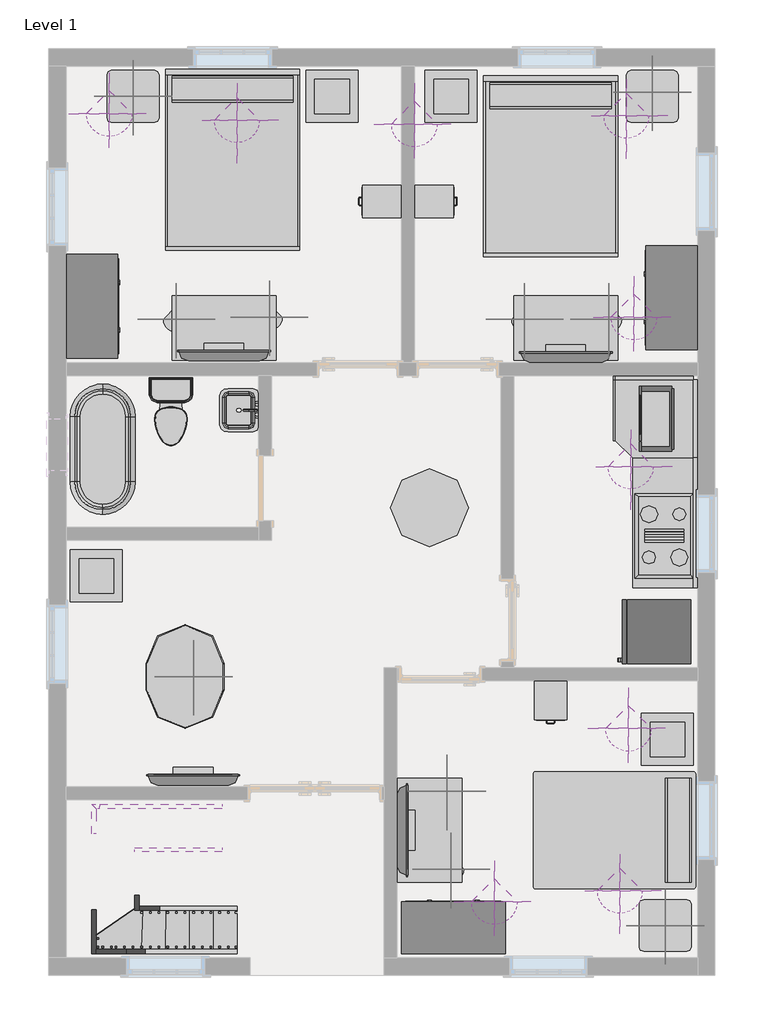
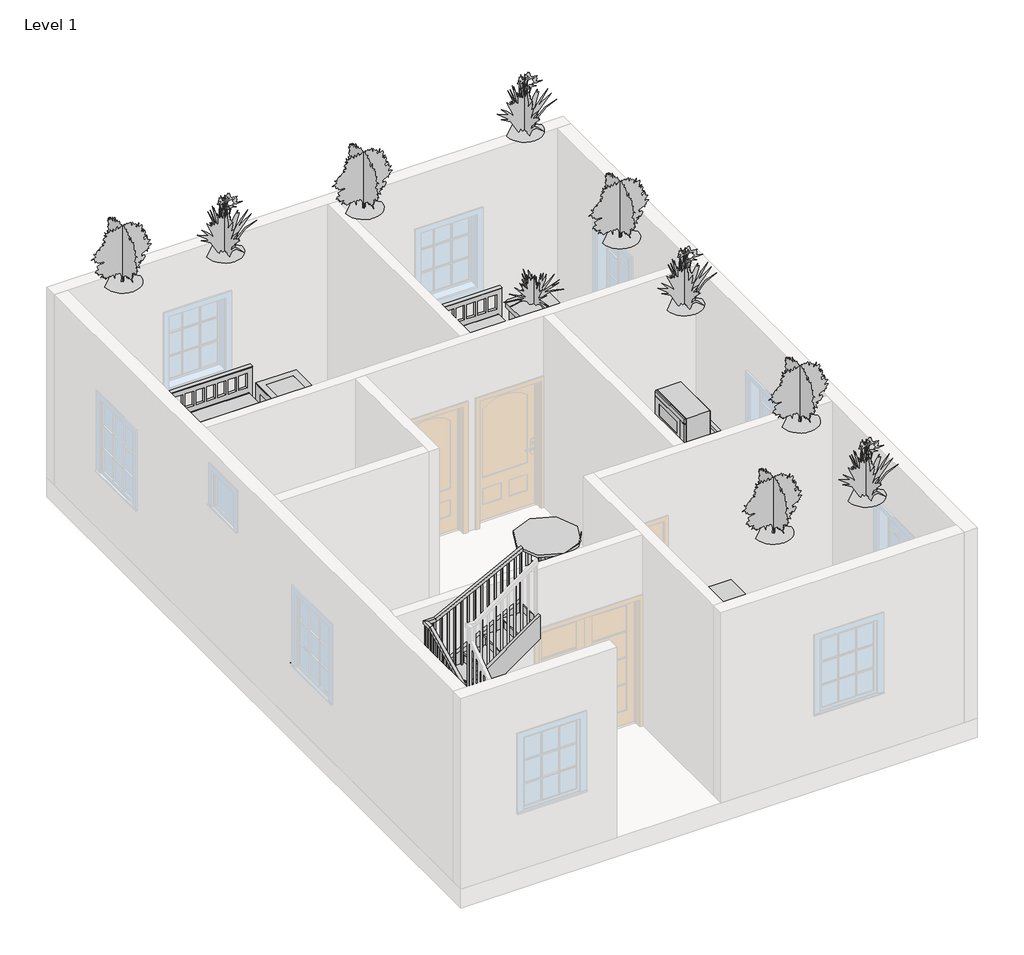
# One storey, part 2 of 2: 26 furniture elements, 19 geographic elements, 9 members, 4 flow terminals, 3 proxies, 1 railing, 1 stair flight.
# Revit data of these elements (continued)
# Elements 8, 9 (IfcFurniture, "Bed-Shaker : Queen 62\" x 83\"") (continued)
#   Materials on its faces: "Birch", "Sash"
# Element 10 (IfcFurniture, "Bed-Standard.0001 : Double 54\" x 75\"")
#   Phase Created = New Construction
#   Materials on its faces: "Linen, White", "Steel, Chrome Plated"
# Elements 11, 12, 13 (IfcFurniture, "Cabinet-File 2 Drawer : 15\" x 18\"")
#   Phase Created = New Construction
#   Materials on its faces: "Steel, Chrome Plated", "Wood - Teak"
# Elements 14, 15, 16 (IfcFurniture, "Dresser : 48\" x 72\" x 24\"")
#   Phase Created = New Construction
#   Materials on its faces: "Laminate, Ivory, Matte", "Cherry", "Wood - Teak"
# Elements 17, 18, 19, 20 (IfcFurniture, "TV - Flat Screen : 42\"")
#   Stand = yes
#   Phase Created = New Construction
#   Materials on its faces: "TV - Black", "TV - Glass", "TV - Screen"
# Elements 21, 22, 23, 24 (IfcFurniture, "Table-Coffee : 24\" x 24\" x 24\"")
#   Phase Created = New Construction
#   Materials on its faces: "Wood", "Glass - Clear, Grey"
# Element 25 (IfcFurniture, "Table-Dining Oval : 36\" x 48\"")
#   Phase Created = New Construction
#   Materials on its faces: "Steel, Chrome Plated", "Glass - Clear, Grey", "Glass"
# Element 26 (IfcFurniture, "Table-Dining Round w Chairs : 36\" Diameter")
#   Phase Created = New Construction
#   Materials on its faces: "Pine", "Laminate, Linen, Matte"
# Elements 27, 28, 29 (IfcFurniture, "Table-End : 24\" x 24\"")
#   Phase Created = New Construction
#   Materials on its faces: "Laminate, Ivory, Matte", "Birch"
# Elements 30, 31, 32 (IfcFurniture, "Table-Rectangular : 72\" x 30\"")
#   Phase Created = New Construction
#   Materials on its faces: "Birch"
# Element 33 (IfcFurniture, "Work Station Cubicle : 96\" x 96\"")
#   Phase Created = New Construction
#   Materials on its faces: "Textile - Light Gray", "Laminate, Ivory, Matte"
# Elements 34, 35, 36, 37 (IfcGeographicElement, "RPC Plant - Tropical")
#   Phase Created = New Construction
# Elements 38, 39, 40, 41, 42, 43, 44, 45, 46, 47 (IfcGeographicElement, "RPC Plant - Tropical : Agave - 1.5'")
#   Phase Created = New Construction
# Elements 48, 49, 50, 51, 52 (IfcGeographicElement, "RPC Plant - Tropical : Jungle Flame - 3'")
#   Phase Created = New Construction
# Elements 53, 54, 55, 56, 57, 58, 59, 60, 61 (IfcMember, "Stringer - 2\" Width")
#   Phase Created = New Construction
# Element 62 (IfcRailing, "Handrail - Rectangular")
#   Phase Created = New Construction
# Element 63 (IfcStairFlight, "2\" Tread 1\" Nosing 1/4\" Riser")
#   Phase Created = New Construction
# Materials
#   "Steel, Chrome Plated": class "Metal", colour RGB 17 17 17, transparency 0, Description = "Chromiuim plated steel", Cost = 0
#   "Steel, Polished": class "Metal", colour RGB 57 57 57, transparency 0, Description = "Polished steel", Cost = 0
#   "Laminate, Linen, Matte": class "Plastic", colour RGB 249 239 230, transparency 0, Description = "Plastic Laminate - Linen, Matte", Cost = 0
#   "Carpet (1)": class "Carpet", colour RGB 124 80 67, transparency 0, Description = "Interior finish"
#   "Porcelain, Linen": class "Ceramic", colour RGB 249 239 230, transparency 0, Description = "Porcelain, linen", Cost = 0
#   "Porcelain, Ivory": class "Ceramic", colour RGB 247 247 239, transparency 0, Description = "Porcelain, ivory", Cost = 0
#   "Birch": class "Wood", colour RGB 224 178 126, transparency 0, Description = "Betula Alleghaniensis", Cost = 0
#   "Sash": class "Wood", colour RGB 224 178 126, transparency 0
#   "Wood - Teak": class "Wood", colour RGB 145 112 90, transparency 0
#   "Cherry": class "Wood", colour RGB 226 177 128, transparency 0, Description = "Prunus Serotina", Cost = 0
#   "Wood": class "Wood", colour RGB 0 0 0, transparency 0, Description = "Generic wood", Cost = 0
#   "Glass": class "Glass", colour RGB 0 128 192, transparency 0.75, Description = "Soda Lime Glass", Cost = 0
#   "Pine": class "Wood", colour RGB 223 192 134, transparency 0, Description = "Pinus Echinata", Cost = 0
#   "Laminate, Ivory, Matte": class "Plastic", colour RGB 247 247 239, transparency 0, Description = "Plastic Laminate - Ivory, Matte", Cost = 0
#   "Textile - Light Gray": class "Fabric", colour RGB 204 204 204, transparency 0
#   "Linen, White": class "Textile", colour RGB 247 247 239, transparency 0, Description = "Linen, white", Cost = 0
#   "TV - Black": colour RGB 49 49 49, transparency 0
#   "TV - Glass": colour RGB 157 157 157, transparency 0.9
#   "TV - Screen": colour RGB 0 0 0, transparency 0
#   "Glass - Clear, Grey": class "Glass", colour RGB 252 255 255, transparency 0.64
